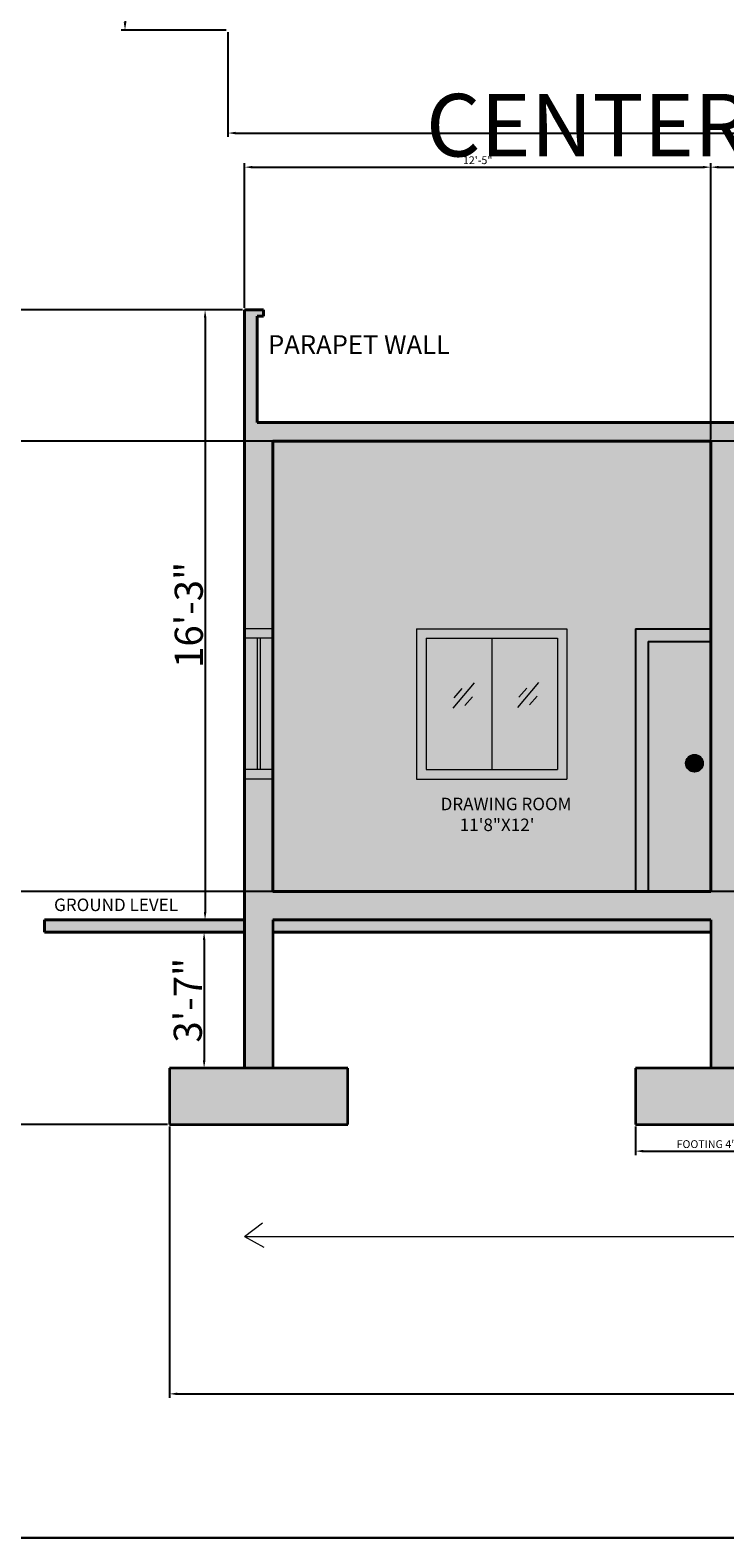
# Model space of a CAD drawing. Units: inches. Extents: x 2163 to 7246, y 928 to 2098.
# Tile 5 of 15: x 2706 to 2928, y 928 to 1411. Entities that reach past the tile are written whole.
import ezdxf

# ---------------------------------------------------------------- set-up
doc = ezdxf.new("R2010")
doc.units = ezdxf.units.IN
for name, color, linetype, lineweight in [('A-ANNO-DIMS', 4, 'Continuous', 18), ('A-ANNO-TEXT', 7, 'Continuous', 18), ('A-ANNO-TITL', 4, 'Continuous', 30), ('A-ANNO-TTLB', 7, 'Continuous', 30), ('A-AREA-IDEN', 7, 'Continuous', 18), ('A-DOOR', 4, 'Continuous', 25), ('A-DOOR-PATT', 35, 'Continuous', 9), ('A-GLAZ', 30, 'Continuous', 20), ('A-SECT', 7, 'Continuous', 40), ('A-SECT-CUT-PATT', 250, 'Continuous', 13), ('S-FNDN', 7, 'Continuous', 35), ('S-FNDN-PATT', 252, 'Continuous', 13)]:
    doc.layers.add(name, color=color, linetype=linetype, lineweight=lineweight)
doc.layers.add('A-GLAZ-PATT', color=141, linetype='Continuous', lineweight=9, true_color=0xadddf7)
doc.layers.add('A-SECT-PATT', color=51, linetype='Continuous', lineweight=9, true_color=0xf8f6b0)
doc.styles.get("Standard").update_dxf_attribs({"font": 'arial.ttf'})
doc.dimstyles.new('ISO-25', dxfattribs={"dimtxt": 2.5, "dimasz": 2.5, "dimexe": 1.25, "dimexo": 0.625, "dimtad": 1, "dimdec": 0, "dimlunit": 3, "dimtxsty": 'Standard', "dimcen": 2.5, "dimadec": 0, "dimazin": 0, "dimtfac": 1, "dimtdec": 0, "dimtmove": 0, "dimatfit": 3, "dimfxl": 1, "dimarcsym": 0})

# ---------------------------------------------------------------- blocks, each defined once
blk = doc.blocks.new('*D27')
at = {"layer": 'A-ANNO-DIMS', "color": 0, "lineweight": -2, "transparency": 16777216}
for p, q in [((2773.92, 1321.11), (2760.66, 1321.11)), ((2761.91, 1318.61), (2761.91, 1128.61)), ((2773.92, 1126.11), (2760.66, 1126.11))]:
    blk.add_line(p, q, dxfattribs=at)
at = {"layer": 'A-ANNO-DIMS', "color": 0, "transparency": 16777216}
for points in [[(2761.5, 1318.61), (2762.33, 1318.61), (2761.91, 1321.11)], [(2761.5, 1128.61), (2762.33, 1128.61), (2761.91, 1126.11)]]:
    blk.add_solid(points, dxfattribs=at)
at = {"layer": 'Defpoints', "color": 0, "transparency": 16777216}
for p in [(2774.54, 1321.11), (2761.91, 1126.11), (2774.54, 1126.11)]:
    blk.add_point(p, dxfattribs=at)
at = {"layer": 'A-ANNO-DIMS', "color": 0, "transparency": 16777216, "insert": (2756.69, 1223.61), "char_height": 2.5, "attachment_point": 5, "rotation": 90}
blk.add_mtext('{\\H3.6x;16\'-3"}', dxfattribs=at)
blk = doc.blocks.new('*D29')
at = {"layer": 'A-ANNO-DIMS', "color": 0, "lineweight": -2, "transparency": 16777216}
for p, q in [((2773.92, 1122.11), (2760.35, 1122.11)), ((2761.6, 1119.61), (2761.6, 1081.18)), ((2773.92, 1078.68), (2760.35, 1078.68))]:
    blk.add_line(p, q, dxfattribs=at)
at = {"layer": 'A-ANNO-DIMS', "color": 0, "transparency": 16777216}
for points in [[(2761.18, 1119.61), (2762.02, 1119.61), (2761.6, 1122.11)], [(2761.18, 1081.18), (2762.02, 1081.18), (2761.6, 1078.68)]]:
    blk.add_solid(points, dxfattribs=at)
at = {"layer": 'Defpoints', "color": 0, "transparency": 16777216}
for p in [(2774.54, 1122.11), (2761.6, 1078.68), (2774.54, 1078.68)]:
    blk.add_point(p, dxfattribs=at)
at = {"layer": 'A-ANNO-DIMS', "color": 0, "transparency": 16777216, "insert": (2756.38, 1100.39), "char_height": 2.5, "attachment_point": 5, "rotation": 90}
blk.add_mtext('{\\H3.6x;3\'-7"}', dxfattribs=at)
blk = doc.blocks.new('FOOTING-57X18-SECTION')
for p, q in [((24, 18), (0, 18)), ((0, 18), (0, 0)), ((57, 18), (24, 18)), ((57, 0), (57, 18)), ((0, 0), (24, 0)), ((24, 0), (57, 0))]:
    blk.add_line(p, q)
blk = doc.blocks.new('DOOR-FRAME-SECTION')
for p, q in [((0, 84), (0, 0)), ((0, 84), (24, 84)), ((4, 80), (24, 80)), ((4, 80), (4, 0))]:
    blk.add_line(p, q)
blk = doc.blocks.new('GLAZ-REFLECTION-SECTION')
for p, q in [((0, 0), (6.77, 8.07)), ((0.29, 3.36), (2.9, 6.25)), ((3.76, 0.92), (6.2, 3.64))]:
    blk.add_line(p, q)
blk = doc.blocks.new('*D55')
at = {"layer": 'A-ANNO-DIMS', "color": 0, "lineweight": -2, "transparency": 16777216}
for p, q in [((2899.54, 1060.06), (2899.54, 1050.88)), ((2956.54, 1060.06), (2956.54, 1050.88)), ((2902.04, 1052.13), (2954.04, 1052.13))]:
    blk.add_line(p, q, dxfattribs=at)
at = {"layer": 'A-ANNO-DIMS', "color": 0, "transparency": 16777216}
for points in [[(2902.04, 1052.55), (2902.04, 1051.71), (2899.54, 1052.13)], [(2954.04, 1052.55), (2954.04, 1051.71), (2956.54, 1052.13)]]:
    blk.add_solid(points, dxfattribs=at)
at = {"layer": 'Defpoints', "color": 0, "transparency": 16777216}
for p in [(2899.54, 1060.68), (2956.54, 1060.68), (2956.54, 1052.13)]:
    blk.add_point(p, dxfattribs=at)
at = {"layer": 'A-ANNO-DIMS', "color": 0, "transparency": 16777216, "insert": (2928.04, 1054.05), "char_height": 2.5, "attachment_point": 5}
blk.add_mtext('FOOTING 4\'-9" TYP.', dxfattribs=at)
blk = doc.blocks.new('*D79')
at = {"layer": 'A-ANNO-DIMS', "color": 0, "lineweight": -2, "transparency": 16777216}
for p, q in [((2769.22, 1409.95), (2769.22, 1376.42)), ((3190.72, 1409.95), (3190.72, 1376.42)), ((2771.72, 1377.67), (3188.22, 1377.67))]:
    blk.add_line(p, q, dxfattribs=at)
at = {"layer": 'A-ANNO-DIMS', "color": 0, "transparency": 16777216}
for points in [[(2771.72, 1378.09), (2771.72, 1377.26), (2769.22, 1377.67)], [(3188.22, 1378.09), (3188.22, 1377.26), (3190.72, 1377.67)]]:
    blk.add_solid(points, dxfattribs=at)
at = {"layer": 'Defpoints', "color": 0, "transparency": 16777216}
for p in [(2769.22, 1410.57), (3190.72, 1410.57), (3190.72, 1377.67)]:
    blk.add_point(p, dxfattribs=at)
at = {"layer": 'A-ANNO-DIMS', "color": 0, "transparency": 16777216, "insert": (2979.97, 1379.59), "char_height": 2.5, "attachment_point": 5}
blk.add_mtext('35\'-1 1/2"', dxfattribs=at)
blk = doc.blocks.new('*D80')
at = {"layer": 'A-ANNO-DIMS', "color": 0, "lineweight": -2, "transparency": 16777216}
for p, q in [((2768.6, 2013.57), (2735.07, 2013.57)), ((2736.32, 2011.07), (2736.32, 1413.07)), ((2768.6, 1410.57), (2735.07, 1410.57))]:
    blk.add_line(p, q, dxfattribs=at)
at = {"layer": 'A-ANNO-DIMS', "color": 0, "transparency": 16777216}
for points in [[(2735.91, 2011.07), (2736.74, 2011.07), (2736.32, 2013.57)], [(2735.91, 1413.07), (2736.74, 1413.07), (2736.32, 1410.57)]]:
    blk.add_solid(points, dxfattribs=at)
at = {"layer": 'Defpoints', "color": 0, "transparency": 16777216}
for p in [(2769.22, 2013.57), (2736.32, 1410.57), (2769.22, 1410.57)]:
    blk.add_point(p, dxfattribs=at)
at = {"layer": 'A-ANNO-DIMS', "color": 0, "transparency": 16777216, "insert": (2734.42, 1712.07), "char_height": 2.5, "attachment_point": 5, "rotation": 90}
blk.add_mtext('50\'-3"', dxfattribs=at)
blk = doc.blocks.new('*D100')
at = {"layer": 'A-ANNO-DIMS', "color": 0, "lineweight": -2, "transparency": 16777216}
for p, q in [((2750.54, 1060.06), (2750.54, 973.27)), ((3539.54, 1060.06), (3539.54, 973.27)), ((2753.04, 974.52), (3537.04, 974.52))]:
    blk.add_line(p, q, dxfattribs=at)
at = {"layer": 'A-ANNO-DIMS', "color": 0, "transparency": 16777216}
for points in [[(2753.04, 974.94), (2753.04, 974.11), (2750.54, 974.52)], [(3537.04, 974.94), (3537.04, 974.11), (3539.54, 974.52)]]:
    blk.add_solid(points, dxfattribs=at)
at = {"layer": 'Defpoints', "color": 0, "transparency": 16777216}
for p in [(2750.54, 1060.68), (3539.54, 1060.68), (3539.54, 974.52)]:
    blk.add_point(p, dxfattribs=at)
at = {"layer": 'A-ANNO-DIMS', "color": 0, "transparency": 16777216, "insert": (3145.04, 976.42), "char_height": 2.5, "attachment_point": 5}
blk.add_mtext('65\'-9"', dxfattribs=at)
blk = doc.blocks.new('*D101')
at = {"layer": 'A-ANNO-DIMS', "color": 0, "lineweight": -2, "transparency": 16777216}
for p, q in [((2773.92, 1321.11), (2663.63, 1321.11)), ((2664.88, 1318.61), (2664.88, 1063.18)), ((2749.92, 1060.68), (2663.63, 1060.68))]:
    blk.add_line(p, q, dxfattribs=at)
at = {"layer": 'A-ANNO-DIMS', "color": 0, "transparency": 16777216}
for points in [[(2664.46, 1318.61), (2665.3, 1318.61), (2664.88, 1321.11)], [(2664.46, 1063.18), (2665.3, 1063.18), (2664.88, 1060.68)]]:
    blk.add_solid(points, dxfattribs=at)
at = {"layer": 'Defpoints', "color": 0, "transparency": 16777216}
for p in [(2774.54, 1321.11), (2664.88, 1060.68), (2750.54, 1060.68)]:
    blk.add_point(p, dxfattribs=at)
at = {"layer": 'A-ANNO-DIMS', "color": 0, "transparency": 16777216, "insert": (2662.96, 1190.89), "char_height": 2.5, "attachment_point": 5, "rotation": 90}
blk.add_mtext('21\'-8 1/2"', dxfattribs=at)
blk = doc.blocks.new('*D102')
at = {"layer": 'A-ANNO-DIMS', "color": 0, "lineweight": -2, "transparency": 16777216}
for p, q in [((2774.54, 1321.73), (2774.54, 1368.01)), ((2777.04, 1366.76), (2921.04, 1366.76)), ((2923.54, 1279.73), (2923.54, 1368.01))]:
    blk.add_line(p, q, dxfattribs=at)
at = {"layer": 'A-ANNO-DIMS', "color": 0, "transparency": 16777216}
for points in [[(2777.04, 1367.17), (2777.04, 1366.34), (2774.54, 1366.76)], [(2921.04, 1367.17), (2921.04, 1366.34), (2923.54, 1366.76)]]:
    blk.add_solid(points, dxfattribs=at)
at = {"layer": 'Defpoints', "color": 0, "transparency": 16777216}
for p in [(2923.54, 1366.76), (2774.54, 1321.11), (2923.54, 1279.11)]:
    blk.add_point(p, dxfattribs=at)
at = {"layer": 'A-ANNO-DIMS', "color": 0, "transparency": 16777216, "insert": (2849.04, 1368.66), "char_height": 2.5, "attachment_point": 5}
blk.add_mtext('12\'-5"', dxfattribs=at)
blk = doc.blocks.new('*D103')
at = {"layer": 'A-ANNO-DIMS', "color": 0, "lineweight": -2, "transparency": 16777216}
for p, q in [((2923.54, 1279.73), (2923.54, 1368.01)), ((2926.04, 1366.76), (3117.04, 1366.76)), ((3119.54, 1279.73), (3119.54, 1368.01))]:
    blk.add_line(p, q, dxfattribs=at)
at = {"layer": 'A-ANNO-DIMS', "color": 0, "transparency": 16777216}
for points in [[(2926.04, 1367.17), (2926.04, 1366.34), (2923.54, 1366.76)], [(3117.04, 1367.17), (3117.04, 1366.34), (3119.54, 1366.76)]]:
    blk.add_solid(points, dxfattribs=at)
at = {"layer": 'Defpoints', "color": 0, "transparency": 16777216}
for p in [(3119.54, 1366.76), (2923.54, 1279.11), (3119.54, 1279.11)]:
    blk.add_point(p, dxfattribs=at)
at = {"layer": 'A-ANNO-DIMS', "color": 0, "transparency": 16777216, "insert": (3021.54, 1368.66), "char_height": 2.5, "attachment_point": 5}
blk.add_mtext('16\'-4"', dxfattribs=at)
blk = doc.blocks.new('*D107')
at = {"layer": 'A-ANNO-DIMS', "color": 0, "lineweight": -2, "transparency": 16777216}
for p, q in [((3256.92, 1279.11), (2663.63, 1279.11)), ((2664.88, 1137.61), (2664.88, 1276.61)), ((3256.92, 1135.11), (2663.63, 1135.11))]:
    blk.add_line(p, q, dxfattribs=at)
at = {"layer": 'A-ANNO-DIMS', "color": 0, "transparency": 16777216}
for points in [[(2664.46, 1276.61), (2665.3, 1276.61), (2664.88, 1279.11)], [(2664.46, 1137.61), (2665.3, 1137.61), (2664.88, 1135.11)]]:
    blk.add_solid(points, dxfattribs=at)
at = {"layer": 'Defpoints', "color": 0, "transparency": 16777216}
for p in [(2664.88, 1279.11), (3257.54, 1279.11), (3257.54, 1135.11)]:
    blk.add_point(p, dxfattribs=at)
at = {"layer": 'A-ANNO-DIMS', "color": 0, "transparency": 16777216, "insert": (2662.98, 1207.11), "char_height": 2.5, "attachment_point": 5, "rotation": 90}
blk.add_mtext('12\'-0"', dxfattribs=at)

msp = doc.modelspace()

# ---------------------------------------------------------------- hatches: boundary and pattern name
at = {"layer": 'A-DOOR-PATT'}
h = msp.add_hatch(color=256, dxfattribs=at)
h.dxf.hatch_style = 1
h.paths.add_polyline_path([(3350.54, 1219.11), (3350.54, 1215.11), (3370.54, 1215.11), (3370.54, 1135.11), (3374.54, 1135.11), (3374.54, 1219.11)])
h.paths.add_polyline_path([(3119.54, 1215.11), (3119.54, 1219.11), (3095.54, 1219.11), (3095.54, 1135.11), (3099.54, 1135.11), (3099.54, 1215.11)])
h.paths.add_polyline_path([(2923.54, 1215.11), (2923.54, 1219.11), (2899.54, 1219.11), (2899.54, 1135.11), (2903.54, 1135.11), (2903.54, 1215.11)])
h = msp.add_hatch(color=256, dxfattribs=at)
h.dxf.hatch_style = 1
h.paths.add_polyline_path([(2923.54, 1215.11), (2903.54, 1215.11), (2903.54, 1135.11), (2923.54, 1135.11)])
h.paths.add_polyline_path([(2921.06, 1176.14, -1), (2915.61, 1176.14, -1)], flags=16)
h.paths.add_polyline_path([(2920.22, 1176.14, -1), (2916.45, 1176.14, -1)], flags=0)
h.paths.add_polyline_path([(3099.54, 1135.11), (3119.54, 1135.11), (3119.54, 1215.11), (3099.54, 1215.11)])
h.paths.add_polyline_path([(3118.83, 1176.14, -1), (3113.38, 1176.14, -1)], flags=16)
h.paths.add_polyline_path([(3117.99, 1176.14, -1), (3114.22, 1176.14, -1)], flags=0)
h.paths.add_polyline_path([(3370.54, 1215.11), (3350.54, 1215.11), (3350.54, 1135.11), (3370.54, 1135.11)])
h.paths.add_polyline_path([(3356.37, 1176.14, -1), (3350.92, 1176.14, -1)], flags=16)
h.paths.add_polyline_path([(3355.53, 1176.14, -1), (3351.76, 1176.14, -1)], flags=0)
h = msp.add_hatch(color=256, dxfattribs=at)
h.dxf.hatch_style = 1
h.paths.add_polyline_path([(2915.61, 1176.14, 1), (2921.06, 1176.14, 1)])
h.paths.add_polyline_path([(2920.22, 1176.14, 1), (2916.45, 1176.14, 1)], flags=16)
h = msp.add_hatch(color=256, dxfattribs=at)
h.dxf.hatch_style = 1
h.paths.add_polyline_path([(2916.45, 1176.14, 1), (2920.22, 1176.14, 1)])
at = {"layer": 'A-GLAZ-PATT'}
h = msp.add_hatch(color=256, dxfattribs=at)
h.dxf.hatch_style = 1
h.paths.add_polyline_path([(2779.54, 1216.11), (2778.54, 1216.11), (2778.54, 1174.11), (2779.54, 1174.11)])
h = msp.add_hatch(color=256, dxfattribs=at)
h.dxf.hatch_style = 1
h.paths.add_polyline_path([(2874.54, 1216.11), (2853.54, 1216.11), (2853.54, 1174.11), (2874.54, 1174.11)])
h.paths.add_polyline_path([(2853.54, 1216.11), (2832.54, 1216.11), (2832.54, 1174.11), (2853.54, 1174.11)])
h.paths.add_polyline_path([(3026.04, 1216.11), (2993.04, 1216.11), (2993.04, 1174.11), (3026.04, 1174.11)])
h.paths.add_polyline_path([(3059.04, 1216.11), (3026.04, 1216.11), (3026.04, 1174.11), (3059.04, 1174.11)])
h.paths.add_polyline_path([(3188.54, 1216.11), (3173.54, 1216.11), (3173.54, 1174.11), (3188.54, 1174.11)])
h.paths.add_polyline_path([(3203.54, 1216.11), (3188.54, 1216.11), (3188.54, 1174.11), (3203.54, 1174.11)])
h.paths.add_polyline_path([(3332.54, 1216.11), (3314.54, 1216.11), (3314.54, 1204.11), (3332.54, 1204.11)])
h.paths.add_polyline_path([(3428.54, 1216.11), (3413.54, 1216.11), (3413.54, 1174.11), (3428.54, 1174.11)])
h.paths.add_polyline_path([(3443.54, 1216.11), (3428.54, 1216.11), (3428.54, 1174.11), (3443.54, 1174.11)])
at = {"layer": 'A-SECT-CUT-PATT'}
h = msp.add_hatch(color=256, dxfattribs=at)
h.dxf.hatch_style = 1
h.paths.add_polyline_path([(2783.54, 1279.11), (2923.54, 1279.11), (2923.54, 1135.11), (2783.54, 1135.11), (2783.54, 1171.11), (2774.54, 1171.11), (2774.54, 1078.68), (2783.54, 1078.68), (2783.54, 1126.11), (2923.54, 1126.11), (2923.54, 1078.68), (2932.54, 1078.68), (2932.54, 1126.11), (3119.54, 1126.11), (3119.54, 1078.68), (3128.54, 1078.68), (3128.54, 1126.11), (3248.54, 1126.11), (3248.54, 1078.68), (3257.54, 1078.68), (3257.54, 1126.11), (3341.54, 1126.11), (3341.54, 1078.68), (3350.54, 1078.68), (3350.54, 1126.11), (3506.54, 1126.11), (3506.54, 1078.68), (3515.54, 1078.68), (3515.54, 1321.11), (3511.54, 1321.11), (3509.54, 1321.11), (3509.54, 1319.11), (3511.54, 1319.11), (3511.54, 1285.11), (2778.54, 1285.11), (2778.54, 1319.11), (2780.54, 1319.11), (2780.54, 1321.11), (2778.54, 1321.11), (2774.54, 1321.11), (2774.54, 1219.11), (2783.54, 1219.11)])
h.paths.add_polyline_path([(2932.54, 1279.11), (3119.54, 1279.11), (3119.54, 1135.11), (2932.54, 1135.11)], flags=16)
h.paths.add_polyline_path([(2990.04, 1219.11), (3062.04, 1219.11), (3062.04, 1171.11), (2990.04, 1171.11)], flags=0)
h.paths.add_polyline_path([(2993.04, 1216.11), (3059.04, 1216.11), (3059.04, 1174.11), (2993.04, 1174.11)], flags=0)
h.paths.add_polyline_path([(3118.83, 1176.14, -1), (3113.38, 1176.14, -1)], flags=0)
h.paths.add_polyline_path([(3117.99, 1176.14, -1), (3114.22, 1176.14, -1)], flags=0)
h.paths.add_polyline_path([(3128.54, 1279.11), (3248.54, 1279.11), (3248.54, 1135.11), (3128.54, 1135.11)], flags=16)
h.paths.add_polyline_path([(3170.54, 1219.11), (3206.54, 1219.11), (3206.54, 1171.11), (3170.54, 1171.11)], flags=0)
h.paths.add_polyline_path([(3173.54, 1216.11), (3203.54, 1216.11), (3203.54, 1174.11), (3173.54, 1174.11)], flags=0)
h.paths.add_polyline_path([(3257.54, 1279.11), (3341.54, 1279.11), (3341.54, 1135.11), (3257.54, 1135.11)], flags=16)
h.paths.add_polyline_path([(3257.54, 1159.11), (3265.54, 1159.11), (3265.54, 1157.11), (3265.04, 1157.11), (3265.04, 1156.11), (3266.54, 1156.11), (3266.54, 1155.11), (3265.04, 1155.11), (3265.04, 1147.11), (3269.54, 1147.11), (3269.54, 1148.11), (3290.04, 1148.11), (3290.04, 1147.11), (3290.54, 1147.11), (3290.54, 1145.11), (3290.04, 1145.11, -0.188679), (3279.54, 1139.66), (3279.54, 1137.11), (3279.54, 1136.11), (3280.54, 1136.11), (3280.54, 1135.11), (3258.54, 1135.11), (3258.54, 1136.11), (3259.54, 1136.11), (3259.54, 1137.11), (3278.54, 1137.11), (3278.54, 1139.59, 0.204728), (3290.04, 1145.11), (3265.54, 1145.11), (3263.54, 1143.11), (3258.04, 1143.11), (3258.04, 1157.11), (3257.54, 1157.11)], flags=0)
h.paths.add_polyline_path([(3311.54, 1219.11), (3335.54, 1219.11), (3335.54, 1201.11), (3311.54, 1201.11)], flags=0)
h.paths.add_polyline_path([(3314.54, 1216.11), (3332.54, 1216.11), (3332.54, 1204.11), (3314.54, 1204.11)], flags=0)
h.paths.add_polyline_path([(3350.54, 1279.11), (3506.54, 1279.11), (3506.54, 1135.11), (3350.54, 1135.11)], flags=16)
h.paths.add_polyline_path([(3356.37, 1176.14, -1), (3350.92, 1176.14, -1)], flags=0)
h.paths.add_polyline_path([(3355.53, 1176.14, -1), (3351.76, 1176.14, -1)], flags=0)
h.paths.add_polyline_path([(3410.54, 1219.11), (3446.54, 1219.11), (3446.54, 1171.11), (3410.54, 1171.11)], flags=0)
h.paths.add_polyline_path([(3413.54, 1216.11), (3443.54, 1216.11), (3443.54, 1174.11), (3413.54, 1174.11)], flags=0)
h = msp.add_hatch(color=256, dxfattribs=at)
h.dxf.hatch_style = 1
h.paths.add_polyline_path([(2783.54, 1216.11), (2783.54, 1219.11), (2774.54, 1219.11), (2774.54, 1216.11)])
h.paths.add_polyline_path([(2774.54, 1174.11), (2774.54, 1171.11), (2783.54, 1171.11), (2783.54, 1174.11)])
h.paths.add_polyline_path([(2877.54, 1171.11), (2877.54, 1219.11), (2829.54, 1219.11), (2829.54, 1171.11)])
h.paths.add_polyline_path([(2832.54, 1174.11), (2832.54, 1216.11), (2874.54, 1216.11), (2874.54, 1174.11)], flags=16)
h.paths.add_polyline_path([(3062.04, 1171.11), (3062.04, 1219.11), (2990.04, 1219.11), (2990.04, 1171.11)])
h.paths.add_polyline_path([(2993.04, 1174.11), (2993.04, 1216.11), (3059.04, 1216.11), (3059.04, 1174.11)], flags=16)
h.paths.add_polyline_path([(3206.54, 1171.11), (3206.54, 1219.11), (3170.54, 1219.11), (3170.54, 1171.11)])
h.paths.add_polyline_path([(3173.54, 1174.11), (3173.54, 1216.11), (3203.54, 1216.11), (3203.54, 1174.11)], flags=16)
h.paths.add_polyline_path([(3335.54, 1201.11), (3335.54, 1219.11), (3311.54, 1219.11), (3311.54, 1201.11)])
h.paths.add_polyline_path([(3314.54, 1204.11), (3314.54, 1216.11), (3332.54, 1216.11), (3332.54, 1204.11)], flags=16)
h.paths.add_polyline_path([(3446.54, 1171.11), (3446.54, 1219.11), (3410.54, 1219.11), (3410.54, 1171.11)])
h.paths.add_polyline_path([(3413.54, 1174.11), (3413.54, 1216.11), (3443.54, 1216.11), (3443.54, 1174.11)], flags=16)
h = msp.add_hatch(color=256, dxfattribs=at)
h.dxf.hatch_style = 1
h.paths.add_polyline_path([(2774.54, 1174.11), (2778.54, 1174.11), (2778.54, 1216.11), (2774.54, 1216.11)])
h.paths.add_polyline_path([(2779.54, 1174.11), (2783.54, 1174.11), (2783.54, 1216.11), (2779.54, 1216.11)])
at = {"layer": 'A-SECT-PATT'}
h = msp.add_hatch(color=256, dxfattribs=at)
h.dxf.hatch_style = 1
h.paths.add_polyline_path([(2783.54, 1279.11), (2783.54, 1135.11), (2899.54, 1135.11), (2899.54, 1219.11), (2923.54, 1219.11), (2923.54, 1279.11)])
h.paths.add_polyline_path([(2877.54, 1219.11), (2877.54, 1171.11), (2829.54, 1171.11), (2829.54, 1219.11)], flags=16)
h.paths.add_polyline_path([(2874.54, 1216.11), (2874.54, 1174.11), (2832.54, 1174.11), (2832.54, 1216.11)], flags=0)
h.paths.add_polyline_path([(2932.54, 1279.11), (2932.54, 1135.11), (3095.54, 1135.11), (3095.54, 1219.11), (3119.54, 1219.11), (3119.54, 1279.11)])
h.paths.add_polyline_path([(3062.04, 1219.11), (3062.04, 1171.11), (2990.04, 1171.11), (2990.04, 1219.11)], flags=16)
h.paths.add_polyline_path([(3059.04, 1216.11), (3059.04, 1174.11), (2993.04, 1174.11), (2993.04, 1216.11)], flags=0)
h.paths.add_polyline_path([(3128.54, 1135.11), (3248.54, 1135.11), (3248.54, 1279.11), (3128.54, 1279.11)])
h.paths.add_polyline_path([(3170.54, 1219.11), (3206.54, 1219.11), (3206.54, 1171.11), (3170.54, 1171.11)], flags=16)
h.paths.add_polyline_path([(3173.54, 1216.11), (3203.54, 1216.11), (3203.54, 1174.11), (3173.54, 1174.11)], flags=0)
h.paths.add_polyline_path([(3257.54, 1159.11), (3265.54, 1159.11), (3265.54, 1157.11), (3265.04, 1157.11), (3265.04, 1156.11), (3266.54, 1156.11), (3266.54, 1155.11), (3265.04, 1155.11), (3265.04, 1147.11), (3269.54, 1147.11), (3269.54, 1148.11), (3290.04, 1148.11), (3290.04, 1147.11), (3290.54, 1147.11), (3290.54, 1145.11), (3290.04, 1145.11, -0.188679), (3279.54, 1139.66), (3279.54, 1137.11), (3279.54, 1136.11), (3280.54, 1136.11), (3280.54, 1135.11), (3341.54, 1135.11), (3341.54, 1279.11), (3257.54, 1279.11)])
h.paths.add_polyline_path([(3311.54, 1219.11), (3335.54, 1219.11), (3335.54, 1201.11), (3311.54, 1201.11)], flags=16)
h.paths.add_polyline_path([(3314.54, 1216.11), (3332.54, 1216.11), (3332.54, 1204.11), (3314.54, 1204.11)], flags=0)
h.paths.add_polyline_path([(3350.54, 1279.11), (3350.54, 1219.11), (3374.54, 1219.11), (3374.54, 1135.11), (3506.54, 1135.11), (3506.54, 1279.11)])
h.paths.add_polyline_path([(3446.54, 1219.11), (3446.54, 1171.11), (3410.54, 1171.11), (3410.54, 1219.11)], flags=16)
h.paths.add_polyline_path([(3443.54, 1216.11), (3443.54, 1174.11), (3413.54, 1174.11), (3413.54, 1216.11)], flags=0)
h.paths.add_polyline_path([(2835.76, 1152.2), (2883.7, 1152.2), (2883.7, 1167.12), (2835.76, 1167.12)], flags=24)
h.paths.add_polyline_path([(3019.5, 1152.59), (3045.3, 1152.59), (3045.3, 1167.51), (3019.5, 1167.51)], flags=24)
h.paths.add_polyline_path([(3180.22, 1151.37), (3206.95, 1151.37), (3206.95, 1166.3), (3180.22, 1166.3)], flags=24)
h.paths.add_polyline_path([(3284.73, 1152.43), (3319.02, 1152.43), (3319.02, 1167.36), (3284.73, 1167.36)], flags=24)
h.paths.add_polyline_path([(3421.37, 1151.92), (3452.45, 1151.92), (3452.45, 1166.85), (3421.37, 1166.85)], flags=24)
at = {"layer": 'S-FNDN-PATT'}
h = msp.add_hatch(color=256, dxfattribs=at)
h.dxf.hatch_style = 1
h.paths.add_polyline_path([(2774.54, 1122.11), (2774.54, 1126.11), (2710.53, 1126.11), (2710.53, 1122.11)])
h = msp.add_hatch(color=256, dxfattribs=at)
h.dxf.hatch_style = 1
h.paths.add_polyline_path([(2783.54, 1126.11), (2783.54, 1122.11), (2923.54, 1122.11), (2923.54, 1126.11)])
h.paths.add_polyline_path([(2932.54, 1126.11), (2932.54, 1122.11), (3119.54, 1122.11), (3119.54, 1126.11)])
h.paths.add_polyline_path([(3128.54, 1126.11), (3128.54, 1122.11), (3248.54, 1122.11), (3248.54, 1126.11)])
h.paths.add_polyline_path([(3341.54, 1122.11), (3341.54, 1126.11), (3257.54, 1126.11), (3257.54, 1122.11)])
h.paths.add_polyline_path([(3350.54, 1126.11), (3350.54, 1122.11), (3506.54, 1122.11), (3506.54, 1126.11)])
h = msp.add_hatch(color=256, dxfattribs=at)
h.dxf.hatch_style = 1
h.paths.add_polyline_path([(2807.54, 1060.68), (2807.54, 1078.68), (2774.54, 1078.68), (2750.54, 1078.68), (2750.54, 1060.68), (2774.54, 1060.68)])
h.paths.add_polyline_path([(2923.54, 1060.68), (2956.54, 1060.68), (2956.54, 1078.68), (2923.54, 1078.68), (2899.54, 1078.68), (2899.54, 1060.68)])
h.paths.add_polyline_path([(3119.54, 1060.68), (3152.54, 1060.68), (3152.54, 1078.68), (3119.54, 1078.68), (3095.54, 1078.68), (3095.54, 1060.68)])
h.paths.add_polyline_path([(3248.54, 1078.68), (3224.54, 1078.68), (3224.54, 1060.68), (3248.54, 1060.68), (3281.54, 1060.68), (3281.54, 1078.68)])
h.paths.add_polyline_path([(3374.54, 1060.68), (3374.54, 1078.68), (3341.54, 1078.68), (3317.54, 1078.68), (3317.54, 1060.68), (3341.54, 1060.68)])
h.paths.add_polyline_path([(3539.54, 1060.68), (3539.54, 1078.68), (3506.54, 1078.68), (3482.54, 1078.68), (3482.54, 1060.68), (3506.54, 1060.68)])

# ---------------------------------------------------------------- linework, layer by layer
at = {"layer": 'A-ANNO-DIMS'}
for q in [(2780.22, 1029.17), (3515.54, 1024.87), (2780.72, 1021.44)]:
    msp.add_line((2774.54, 1024.87), q, dxfattribs=at)
at = {"layer": 'A-ANNO-TTLB'}
msp.add_lwpolyline([(2162.62, 2098.21), (3633.38, 2098.21), (3633.38, 928.48), (2162.62, 928.48)], close=True, dxfattribs=at)
at = {"layer": 'A-DOOR'}
for radius in [2.72, 1.89]:
    msp.add_circle((2918.34, 1176.14), radius, dxfattribs=at)
at = {"layer": 'A-GLAZ'}
for p, q in [((2783.54, 1219.11), (2774.54, 1219.11)), ((2783.54, 1216.11), (2774.54, 1216.11)), ((2778.54, 1216.11), (2778.54, 1174.11)), ((2779.54, 1216.11), (2779.54, 1174.11)), ((2829.54, 1219.11), (2877.54, 1219.11)), ((2829.54, 1219.11), (2829.54, 1171.11)), ((2832.54, 1216.11), (2874.54, 1216.11)), ((2832.54, 1216.11), (2832.54, 1174.11)), ((2853.54, 1216.11), (2853.54, 1174.11)), ((2874.54, 1216.11), (2874.54, 1174.11)), ((2877.54, 1219.11), (2877.54, 1171.11)), ((2783.54, 1174.11), (2774.54, 1174.11)), ((2832.54, 1174.11), (2874.54, 1174.11)), ((2783.54, 1171.11), (2774.54, 1171.11)), ((2829.54, 1171.11), (2877.54, 1171.11))]:
    msp.add_line(p, q, dxfattribs=at)
at = {"layer": 'A-SECT'}
for p, q in [((2774.54, 1321.11), (2774.54, 1078.68)), ((2774.54, 1321.11), (2778.54, 1321.11)), ((2778.54, 1321.11), (2780.54, 1321.11)), ((2780.54, 1321.11), (2780.54, 1319.11)), ((2778.54, 1319.11), (2778.54, 1285.11)), ((2780.54, 1319.11), (2778.54, 1319.11)), ((2778.54, 1285.11), (3511.54, 1285.11)), ((2783.54, 1279.11), (2783.54, 1135.11)), ((2783.54, 1279.11), (2923.54, 1279.11)), ((2923.54, 1279.11), (2923.54, 1135.11)), ((2783.54, 1135.11), (2923.54, 1135.11)), ((2710.53, 1126.11), (2774.54, 1126.11)), ((2710.53, 1126.11), (2710.53, 1122.11)), ((2783.54, 1126.11), (2923.54, 1126.11)), ((2710.53, 1122.11), (2774.54, 1122.11)), ((2783.54, 1122.11), (2923.54, 1122.11))]:
    msp.add_line(p, q, dxfattribs=at)
at = {"layer": 'S-FNDN'}
for p, q in [((2783.54, 1126.11), (2783.54, 1078.68)), ((2923.54, 1126.11), (2923.54, 1078.68))]:
    msp.add_line(p, q, dxfattribs=at)

# ---------------------------------------------------------------- block references
at = {"layer": 'A-DOOR'}
msp.add_blockref('DOOR-FRAME-SECTION', (2899.54, 1135.11), dxfattribs=at)
at = {"layer": 'A-GLAZ'}
for p in [(2841.22, 1193.76), (2841.22, 1193.76), (2861.87, 1193.95)]:
    msp.add_blockref('GLAZ-REFLECTION-SECTION', p, dxfattribs=at)
at = {"layer": 'S-FNDN'}
for p in [(2750.54, 1060.68), (2899.54, 1060.68)]:
    msp.add_blockref('FOOTING-57X18-SECTION', p, dxfattribs=at)

# ---------------------------------------------------------------- texts
at = {"layer": 'A-ANNO-TEXT', "attachment_point": 1}
for s, width, insert, char_height in [('PARAPET WALL', 124.931, (2782.04, 1313.03), 6), ('GROUND LEVEL', 292.6399, (2713.63, 1132.89), 4)]:
    msp.add_mtext_dynamic_manual_height_columns(s, width=width, gutter_width=12.5, heights=[0], dxfattribs=dict(at, insert=insert, char_height=char_height))
at = {"layer": 'A-ANNO-TITL', "insert": (2832.54, 1390.19), "char_height": 20, "attachment_point": 1}
msp.add_mtext_dynamic_manual_height_columns('CENTER LINE DIAGRAM', width=571.2399, gutter_width=12.5, heights=[0], dxfattribs=at)
at = {"layer": 'A-AREA-IDEN', "insert": (2837.19, 1165.14), "char_height": 4, "attachment_point": 1}
msp.add_mtext_dynamic_manual_height_columns('DRAWING ROOM\\P     11\'8"X12\'', width=47.6539, gutter_width=12.5, heights=[0], dxfattribs=at)

# ---------------------------------------------------------------- dimensions: what is measured, and where the dimension line sits
at = {"layer": 'A-ANNO-DIMS'}
for base, p1, p2, picture, middle in [((2736.32, 1410.57), (2769.22, 2013.57), (2769.22, 1410.57), '*D80', (2734.42, 1712.07)), ((2664.88, 1060.68), (2774.54, 1321.11), (2750.54, 1060.68), '*D101', (2662.96, 1190.89)), ((2664.88, 1279.11), (3257.54, 1135.11), (3257.54, 1279.11), '*D107', (2662.98, 1207.11))]:
    dim = msp.add_linear_dim(base=base, p1=p1, p2=p2, angle=90, dimstyle='ISO-25', override={"dimdec": 1, "dimlfac": 1, "dimrnd": 0, "dimzin": 1, "dimdsep": 46, "dimlunit": 4, "dimfrac": 2}, dxfattribs=at)
    dim.commit()
    dim.dimension.update_dxf_attribs({"geometry": picture, "text_midpoint": middle})
for base, p1, p2, picture, middle in [((3190.72, 1377.67), (2769.22, 1410.57), (3190.72, 1410.57), '*D79', (2979.97, 1379.59)), ((2923.54, 1366.76), (2774.54, 1321.11), (2923.54, 1279.11), '*D102', (2849.04, 1368.66)), ((3119.54, 1366.76), (2923.54, 1279.11), (3119.54, 1279.11), '*D103', (3021.54, 1368.66)), ((3539.54, 974.52), (2750.54, 1060.68), (3539.54, 1060.68), '*D100', (3145.04, 976.42))]:
    dim = msp.add_linear_dim(base=base, p1=p1, p2=p2, dimstyle='ISO-25', override={"dimdec": 1, "dimlfac": 1, "dimrnd": 0, "dimzin": 1, "dimdsep": 46, "dimlunit": 4, "dimfrac": 2}, dxfattribs=at)
    dim.commit()
    dim.dimension.update_dxf_attribs({"geometry": picture, "text_midpoint": middle})
dim = msp.add_linear_dim(base=(2761.91, 1126.11), p1=(2774.54, 1321.11), p2=(2774.54, 1126.11), angle=90, text='{\\H3.6x;<>}', dimstyle='ISO-25', override={"dimclrd": 0, "dimclre": 0, "dimclrt": 0}, dxfattribs=at)
dim.commit()
dim.dimension.update_dxf_attribs({"geometry": '*D27', "text_midpoint": (2761.91, 1223.61), "dimtype": 160})
dim = msp.add_linear_dim(base=(2761.6, 1078.68), p1=(2774.54, 1122.11), p2=(2774.54, 1078.68), angle=90, text='{\\H3.6x;<>}', dimstyle='ISO-25', override={"dimclrd": 0, "dimclre": 0, "dimclrt": 0}, dxfattribs=at)
dim.commit()
dim.dimension.update_dxf_attribs({"geometry": '*D29', "text_midpoint": (2756.38, 1100.39)})
dim = msp.add_linear_dim(base=(2956.54, 1052.13), p1=(2899.54, 1060.68), p2=(2956.54, 1060.68), text='FOOTING <> TYP.', dimstyle='ISO-25', override={"dimdec": 1, "dimlfac": 1, "dimrnd": 0, "dimzin": 1, "dimdsep": 46, "dimlunit": 4, "dimfrac": 2}, dxfattribs=at)
dim.commit()
dim.dimension.update_dxf_attribs({"geometry": '*D55', "text_midpoint": (2928.04, 1054.05)})

doc.saveas('drawing.dxf')
